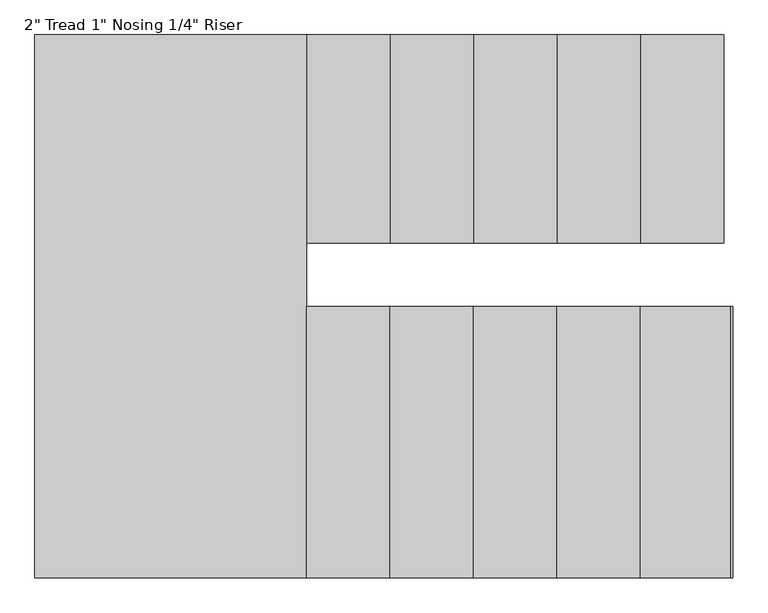
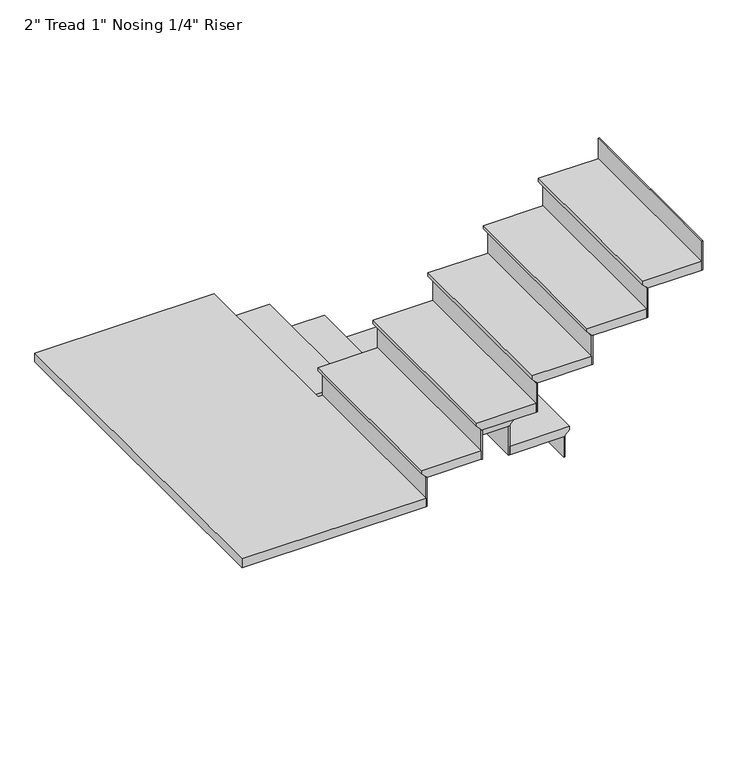
"""IFC4 building model written with IfcOpenShell, lengths in millimetres: stair flight geometry."""

from ifc_helpers import new_model, si_unit, origin, place, context, project, spatial, faceted_brep, source, transform, mapped, element, save


def stair_flight_8724fc67(model_context):
    return source(origin(), model_context, "Body", "Brep", [
        faceted_brep([(-3084.0415084, -317.1427733, 3350.6833333), (-3084.0415084, -317.1427733, 3369.7333333), (-3084.0415084, -1076.6758739, 3369.7333333), (-3084.0415084, -1076.6758739, 3350.6833333), (-3109.4415084, -317.1427733, 3325.2833333), (-3109.4415084, -1076.6758739, 3325.2833333), (-3414.2415084, -317.1427733, 3369.7333333), (-3414.2415084, -1076.6758739, 3369.7333333), (-3109.4415084, -1076.6758739, 3318.9333333), (-3414.2415084, -1076.6758739, 3318.9333333), (-3414.2415084, -317.1427733, 3318.9333333), (-3109.4415084, -317.1427733, 3318.9333333)], [[[0, 1, 2, 3]], [[4, 0, 3, 5]], [[2, 1, 6, 7]], [[8, 9, 10, 11]], [[2, 7, 9, 8, 5, 3]], [[8, 11, 4, 5]], [[6, 1, 0, 4, 11, 10]], [[7, 6, 10, 9]]]),
        faceted_brep([(-3109.4415084, -317.1427733, 3318.9333333), (-3109.4415084, -317.1427733, 3200.4), (-3115.7915084, -317.1427733, 3200.4), (-3115.7915084, -317.1427733, 3318.9333333), (-3109.4415084, -1076.6758739, 3318.9333333), (-3115.7915084, -1076.6758739, 3318.9333333), (-3115.7915084, -1076.6758739, 3200.4), (-3109.4415084, -1076.6758739, 3200.4)], [[[0, 1, 2, 3]], [[4, 5, 6, 7]], [[1, 0, 4, 7]], [[2, 1, 7, 6]], [[3, 2, 6, 5]], [[0, 3, 5, 4]]]),
        faceted_brep([(-3414.2415084, -317.1427733, 3488.2666667), (-3414.2415084, -317.1427733, 3318.9333333), (-3420.5915084, -317.1427733, 3318.9333333), (-3420.5915084, -317.1427733, 3488.2666667), (-3414.2415084, -1076.6758739, 3488.2666667), (-3420.5915084, -1076.6758739, 3488.2666667), (-3420.5915084, -1076.6758739, 3318.9333333), (-3414.2415084, -1076.6758739, 3318.9333333)], [[[0, 1, 2, 3]], [[4, 5, 6, 7]], [[1, 0, 4, 7]], [[2, 1, 7, 6]], [[3, 2, 6, 5]], [[0, 3, 5, 4]]]),
        faceted_brep([(-3388.8415084, -1076.6758739, 3539.0666667), (-3388.8415084, -317.1427733, 3539.0666667), (-3719.0415084, -317.1427733, 3539.0666667), (-3719.0415084, -1076.6758739, 3539.0666667), (-3414.2415084, -1076.6758739, 3488.2666667), (-3719.0415084, -1076.6758739, 3488.2666667), (-3719.0415084, -317.1427733, 3488.2666667), (-3414.2415084, -317.1427733, 3488.2666667), (-3414.2415084, -1076.6758739, 3494.6166667), (-3388.8415084, -1076.6758739, 3520.0166667), (-3414.2415084, -317.1427733, 3494.6166667), (-3388.8415084, -317.1427733, 3520.0166667)], [[[0, 1, 2, 3]], [[4, 5, 6, 7]], [[0, 3, 5, 4, 8, 9]], [[4, 7, 10, 8]], [[2, 1, 11, 10, 7, 6]], [[3, 2, 6, 5]], [[11, 1, 0, 9]], [[10, 11, 9, 8]]]),
        faceted_brep([(-3719.0415084, -317.1427733, 3657.6), (-3719.0415084, -317.1427733, 3488.2666667), (-3725.3915084, -317.1427733, 3488.2666667), (-3725.3915084, -317.1427733, 3657.6), (-3719.0415084, -1076.6758739, 3657.6), (-3725.3915084, -1076.6758739, 3657.6), (-3725.3915084, -1076.6758739, 3488.2666667), (-3719.0415084, -1076.6758739, 3488.2666667)], [[[0, 1, 2, 3]], [[4, 5, 6, 7]], [[1, 0, 4, 7]], [[2, 1, 7, 6]], [[3, 2, 6, 5]], [[0, 3, 5, 4]]]),
        faceted_brep([(-3693.6415084, -1076.6758739, 3708.4), (-3693.6415084, -317.1427733, 3708.4), (-4023.8415084, -317.1427733, 3708.4), (-4023.8415084, -1076.6758739, 3708.4), (-3719.0415084, -1076.6758739, 3657.6), (-4023.8415084, -1076.6758739, 3657.6), (-4023.8415084, -317.1427733, 3657.6), (-3719.0415084, -317.1427733, 3657.6), (-3719.0415084, -1076.6758739, 3663.95), (-3693.6415084, -1076.6758739, 3689.35), (-3719.0415084, -317.1427733, 3663.95), (-3693.6415084, -317.1427733, 3689.35)], [[[0, 1, 2, 3]], [[4, 5, 6, 7]], [[0, 3, 5, 4, 8, 9]], [[4, 7, 10, 8]], [[2, 1, 11, 10, 7, 6]], [[3, 2, 6, 5]], [[11, 1, 0, 9]], [[10, 11, 9, 8]]]),
        faceted_brep([(-4023.8415084, -317.1427733, 3826.9333333), (-4023.8415084, -317.1427733, 3657.6), (-4030.1915084, -317.1427733, 3657.6), (-4030.1915084, -317.1427733, 3826.9333333), (-4023.8415084, -1076.6758739, 3826.9333333), (-4030.1915084, -1076.6758739, 3826.9333333), (-4030.1915084, -1076.6758739, 3657.6), (-4023.8415084, -1076.6758739, 3657.6)], [[[0, 1, 2, 3]], [[4, 5, 6, 7]], [[1, 0, 4, 7]], [[2, 1, 7, 6]], [[3, 2, 6, 5]], [[0, 3, 5, 4]]]),
        faceted_brep([(-3998.4415084, -1076.6758739, 3877.7333333), (-3998.4415084, -317.1427733, 3877.7333333), (-4328.6415084, -317.1427733, 3877.7333333), (-4328.6415084, -1076.6758739, 3877.7333333), (-4023.8415084, -1076.6758739, 3826.9333333), (-4328.6415084, -1076.6758739, 3826.9333333), (-4328.6415084, -317.1427733, 3826.9333333), (-4023.8415084, -317.1427733, 3826.9333333), (-4023.8415084, -1076.6758739, 3833.2833333), (-3998.4415084, -1076.6758739, 3858.6833333), (-4023.8415084, -317.1427733, 3833.2833333), (-3998.4415084, -317.1427733, 3858.6833333)], [[[0, 1, 2, 3]], [[4, 5, 6, 7]], [[0, 3, 5, 4, 8, 9]], [[4, 7, 10, 8]], [[2, 1, 11, 10, 7, 6]], [[3, 2, 6, 5]], [[11, 1, 0, 9]], [[10, 11, 9, 8]]]),
        faceted_brep([(-4328.6415084, -317.1427733, 3996.2666667), (-4328.6415084, -317.1427733, 3826.9333333), (-4334.9915084, -317.1427733, 3826.9333333), (-4334.9915084, -317.1427733, 3996.2666667), (-4328.6415084, -1076.6758739, 3996.2666667), (-4334.9915084, -1076.6758739, 3996.2666667), (-4334.9915084, -1076.6758739, 3826.9333333), (-4328.6415084, -1076.6758739, 3826.9333333)], [[[0, 1, 2, 3]], [[4, 5, 6, 7]], [[1, 0, 4, 7]], [[2, 1, 7, 6]], [[3, 2, 6, 5]], [[0, 3, 5, 4]]]),
        faceted_brep([(-4303.2415084, -1076.6758739, 4047.0666667), (-4303.2415084, -317.1427733, 4047.0666667), (-4633.4415084, -317.1427733, 4047.0666667), (-4633.4415084, -1076.6758739, 4047.0666667), (-4328.6415084, -1076.6758739, 3996.2666667), (-4633.4415084, -1076.6758739, 3996.2666667), (-4633.4415084, -317.1427733, 3996.2666667), (-4328.6415084, -317.1427733, 3996.2666667), (-4328.6415084, -1076.6758739, 4002.6166667), (-4303.2415084, -1076.6758739, 4028.0166667), (-4328.6415084, -317.1427733, 4002.6166667), (-4303.2415084, -317.1427733, 4028.0166667)], [[[0, 1, 2, 3]], [[4, 5, 6, 7]], [[0, 3, 5, 4, 8, 9]], [[4, 7, 10, 8]], [[2, 1, 11, 10, 7, 6]], [[3, 2, 6, 5]], [[11, 1, 0, 9]], [[10, 11, 9, 8]]]),
        faceted_brep([(-4633.4415084, -317.1427733, 4165.6), (-4633.4415084, -317.1427733, 3996.2666667), (-4639.7915084, -317.1427733, 3996.2666667), (-4639.7915084, -317.1427733, 4165.6), (-4633.4415084, -1076.6758739, 4165.6), (-4639.7915084, -1076.6758739, 4165.6), (-4639.7915084, -1076.6758739, 3996.2666667), (-4633.4415084, -1076.6758739, 3996.2666667)], [[[0, 1, 2, 3]], [[4, 5, 6, 7]], [[1, 0, 4, 7]], [[2, 1, 7, 6]], [[3, 2, 6, 5]], [[0, 3, 5, 4]]]),
        faceted_brep([(-4582.6415084, -1307.7427733, 4216.4), (-4608.0415084, -1307.7427733, 4216.4), (-4608.0415084, -317.1427733, 4216.4), (-5598.6415084, -317.1427733, 4216.4), (-5598.6415084, -2298.3427733, 4216.4), (-4582.6415084, -2298.3427733, 4216.4), (-4608.0415084, -1307.7427733, 4165.6), (-4582.6415084, -1307.7427733, 4165.6), (-4582.6415084, -2298.3427733, 4165.6), (-5598.6415084, -2298.3427733, 4165.6), (-5598.6415084, -317.1427733, 4165.6), (-4633.4415084, -317.1427733, 4165.6), (-4633.4415084, -1076.6758739, 4165.6), (-4608.0415084, -1076.6758739, 4165.6), (-4608.0415084, -1076.6758739, 4197.35), (-4608.0415084, -317.1427733, 4197.35), (-4633.4415084, -1076.6758739, 4171.95), (-4633.4415084, -317.1427733, 4171.95)], [[[0, 1, 2, 3, 4, 5]], [[6, 7, 8, 9, 10, 11, 12, 13]], [[1, 0, 7, 6]], [[2, 1, 6, 13, 14, 15]], [[13, 12, 16, 14]], [[12, 11, 17, 16]], [[3, 2, 15, 17, 11, 10]], [[4, 3, 10, 9]], [[5, 4, 9, 8]], [[0, 5, 8, 7]], [[17, 15, 14, 16]]]),
        faceted_brep([(-4582.6415084, -2298.3427733, 4334.9333333), (-4582.6415084, -2298.3427733, 4165.6), (-4576.2915084, -2298.3427733, 4165.6), (-4576.2915084, -2298.3427733, 4334.9333333), (-4582.6415084, -1307.7427733, 4334.9333333), (-4576.2915084, -1307.7427733, 4334.9333333), (-4576.2915084, -1307.7427733, 4165.6), (-4582.6415084, -1307.7427733, 4165.6)], [[[0, 1, 2, 3]], [[4, 5, 6, 7]], [[1, 0, 4, 7]], [[2, 1, 7, 6]], [[3, 2, 6, 5]], [[0, 3, 5, 4]]]),
        faceted_brep([(-4608.0415084, -1307.7427733, 4385.7333333), (-4608.0415084, -2298.3427733, 4385.7333333), (-4277.8415084, -2298.3427733, 4385.7333333), (-4277.8415084, -1307.7427733, 4385.7333333), (-4582.6415084, -1307.7427733, 4334.9333333), (-4277.8415084, -1307.7427733, 4334.9333333), (-4277.8415084, -2298.3427733, 4334.9333333), (-4582.6415084, -2298.3427733, 4334.9333333), (-4582.6415084, -1307.7427733, 4341.2833333), (-4608.0415084, -1307.7427733, 4366.6833333), (-4582.6415084, -2298.3427733, 4341.2833333), (-4608.0415084, -2298.3427733, 4366.6833333)], [[[0, 1, 2, 3]], [[4, 5, 6, 7]], [[0, 3, 5, 4, 8, 9]], [[4, 7, 10, 8]], [[2, 1, 11, 10, 7, 6]], [[3, 2, 6, 5]], [[11, 1, 0, 9]], [[10, 11, 9, 8]]]),
        faceted_brep([(-4277.8415084, -2298.3427733, 4504.2666667), (-4277.8415084, -2298.3427733, 4334.9333333), (-4271.4915084, -2298.3427733, 4334.9333333), (-4271.4915084, -2298.3427733, 4504.2666667), (-4277.8415084, -1307.7427733, 4504.2666667), (-4271.4915084, -1307.7427733, 4504.2666667), (-4271.4915084, -1307.7427733, 4334.9333333), (-4277.8415084, -1307.7427733, 4334.9333333)], [[[0, 1, 2, 3]], [[4, 5, 6, 7]], [[1, 0, 4, 7]], [[2, 1, 7, 6]], [[3, 2, 6, 5]], [[0, 3, 5, 4]]]),
        faceted_brep([(-4303.2415084, -1307.7427733, 4555.0666667), (-4303.2415084, -2298.3427733, 4555.0666667), (-3973.0415084, -2298.3427733, 4555.0666667), (-3973.0415084, -1307.7427733, 4555.0666667), (-4277.8415084, -1307.7427733, 4504.2666667), (-3973.0415084, -1307.7427733, 4504.2666667), (-3973.0415084, -2298.3427733, 4504.2666667), (-4277.8415084, -2298.3427733, 4504.2666667), (-4277.8415084, -1307.7427733, 4510.6166667), (-4303.2415084, -1307.7427733, 4536.0166667), (-4277.8415084, -2298.3427733, 4510.6166667), (-4303.2415084, -2298.3427733, 4536.0166667)], [[[0, 1, 2, 3]], [[4, 5, 6, 7]], [[0, 3, 5, 4, 8, 9]], [[4, 7, 10, 8]], [[2, 1, 11, 10, 7, 6]], [[3, 2, 6, 5]], [[11, 1, 0, 9]], [[10, 11, 9, 8]]]),
        faceted_brep([(-3973.0415084, -2298.3427733, 4673.6), (-3973.0415084, -2298.3427733, 4504.2666667), (-3966.6915084, -2298.3427733, 4504.2666667), (-3966.6915084, -2298.3427733, 4673.6), (-3973.0415084, -1307.7427733, 4673.6), (-3966.6915084, -1307.7427733, 4673.6), (-3966.6915084, -1307.7427733, 4504.2666667), (-3973.0415084, -1307.7427733, 4504.2666667)], [[[0, 1, 2, 3]], [[4, 5, 6, 7]], [[1, 0, 4, 7]], [[2, 1, 7, 6]], [[3, 2, 6, 5]], [[0, 3, 5, 4]]]),
        faceted_brep([(-3998.4415084, -1307.7427733, 4724.4), (-3998.4415084, -2298.3427733, 4724.4), (-3668.2415084, -2298.3427733, 4724.4), (-3668.2415084, -1307.7427733, 4724.4), (-3973.0415084, -1307.7427733, 4673.6), (-3668.2415084, -1307.7427733, 4673.6), (-3668.2415084, -2298.3427733, 4673.6), (-3973.0415084, -2298.3427733, 4673.6), (-3973.0415084, -1307.7427733, 4679.95), (-3998.4415084, -1307.7427733, 4705.35), (-3973.0415084, -2298.3427733, 4679.95), (-3998.4415084, -2298.3427733, 4705.35)], [[[0, 1, 2, 3]], [[4, 5, 6, 7]], [[0, 3, 5, 4, 8, 9]], [[4, 7, 10, 8]], [[2, 1, 11, 10, 7, 6]], [[3, 2, 6, 5]], [[11, 1, 0, 9]], [[10, 11, 9, 8]]]),
        faceted_brep([(-3668.2415084, -2298.3427733, 4842.9333333), (-3668.2415084, -2298.3427733, 4673.6), (-3661.8915084, -2298.3427733, 4673.6), (-3661.8915084, -2298.3427733, 4842.9333333), (-3668.2415084, -1307.7427733, 4842.9333333), (-3661.8915084, -1307.7427733, 4842.9333333), (-3661.8915084, -1307.7427733, 4673.6), (-3668.2415084, -1307.7427733, 4673.6)], [[[0, 1, 2, 3]], [[4, 5, 6, 7]], [[1, 0, 4, 7]], [[2, 1, 7, 6]], [[3, 2, 6, 5]], [[0, 3, 5, 4]]]),
        faceted_brep([(-3693.6415084, -1307.7427733, 4893.7333333), (-3693.6415084, -2298.3427733, 4893.7333333), (-3363.4415084, -2298.3427733, 4893.7333333), (-3363.4415084, -1307.7427733, 4893.7333333), (-3668.2415084, -1307.7427733, 4842.9333333), (-3363.4415084, -1307.7427733, 4842.9333333), (-3363.4415084, -2298.3427733, 4842.9333333), (-3668.2415084, -2298.3427733, 4842.9333333), (-3668.2415084, -1307.7427733, 4849.2833333), (-3693.6415084, -1307.7427733, 4874.6833333), (-3668.2415084, -2298.3427733, 4849.2833333), (-3693.6415084, -2298.3427733, 4874.6833333)], [[[0, 1, 2, 3]], [[4, 5, 6, 7]], [[0, 3, 5, 4, 8, 9]], [[4, 7, 10, 8]], [[2, 1, 11, 10, 7, 6]], [[3, 2, 6, 5]], [[11, 1, 0, 9]], [[10, 11, 9, 8]]]),
        faceted_brep([(-3363.4415084, -2298.3427733, 5012.2666667), (-3363.4415084, -2298.3427733, 4842.9333333), (-3357.0915084, -2298.3427733, 4842.9333333), (-3357.0915084, -2298.3427733, 5012.2666667), (-3363.4415084, -1307.7427733, 5012.2666667), (-3357.0915084, -1307.7427733, 5012.2666667), (-3357.0915084, -1307.7427733, 4842.9333333), (-3363.4415084, -1307.7427733, 4842.9333333)], [[[0, 1, 2, 3]], [[4, 5, 6, 7]], [[1, 0, 4, 7]], [[2, 1, 7, 6]], [[3, 2, 6, 5]], [[0, 3, 5, 4]]]),
        faceted_brep([(-3058.6415084, -2298.3427733, 5181.6), (-3058.6415084, -2298.3427733, 5012.2666667), (-3052.2915084, -2298.3427733, 5012.2666667), (-3052.2915084, -2298.3427733, 5181.6), (-3058.6415084, -1307.7427733, 5181.6), (-3052.2915084, -1307.7427733, 5181.6), (-3052.2915084, -1307.7427733, 5012.2666667), (-3058.6415084, -1307.7427733, 5012.2666667)], [[[0, 1, 2, 3]], [[4, 5, 6, 7]], [[1, 0, 4, 7]], [[2, 1, 7, 6]], [[3, 2, 6, 5]], [[0, 3, 5, 4]]]),
        faceted_brep([(-3388.8415084, -1307.7427733, 5063.0666667), (-3388.8415084, -2298.3427733, 5063.0666667), (-3058.6415084, -2298.3427733, 5063.0666667), (-3058.6415084, -1307.7427733, 5063.0666667), (-3363.4415084, -1307.7427733, 5012.2666667), (-3058.6415084, -1307.7427733, 5012.2666667), (-3058.6415084, -2298.3427733, 5012.2666667), (-3363.4415084, -2298.3427733, 5012.2666667), (-3363.4415084, -1307.7427733, 5018.6166667), (-3388.8415084, -1307.7427733, 5044.0166667), (-3363.4415084, -2298.3427733, 5018.6166667), (-3388.8415084, -2298.3427733, 5044.0166667)], [[[0, 1, 2, 3]], [[4, 5, 6, 7]], [[0, 3, 5, 4, 8, 9]], [[4, 7, 10, 8]], [[2, 1, 11, 10, 7, 6]], [[3, 2, 6, 5]], [[11, 1, 0, 9]], [[10, 11, 9, 8]]]),
    ])


if __name__ == "__main__":
    model = new_model("IFC4")
    model_context = context("Model", 3, world=origin())
    ifc_project = project(units=[si_unit("LENGTHUNIT", "METRE", prefix="MILLI")], contexts=[model_context])
    site = spatial("IfcSite", under=ifc_project)
    building = spatial("IfcBuilding", under=site)
    placement = place(None, origin())
    stair_flight_shape = stair_flight_8724fc67(model_context)
    element("IfcStairFlight", 1, ObjectType="2\" Tread 1\" Nosing 1/4\" Riser", at=placement, inside=building, context=model_context, shape_type="MappedRepresentation", body=[
        mapped(stair_flight_shape, transform((0.0, 0.0, 0.0), x_axis=(1.0, 0.0, 0.0), y_axis=(0.0, 1.0, 0.0), z_axis=(0.0, 0.0, 1.0))),
    ])
    save(model, "model.ifc")
